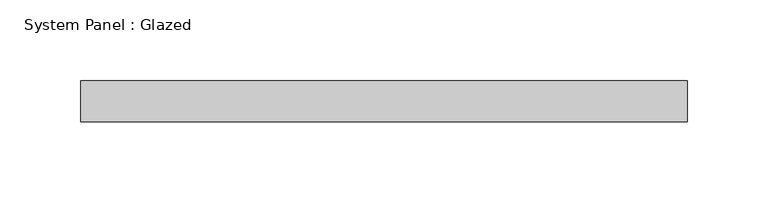
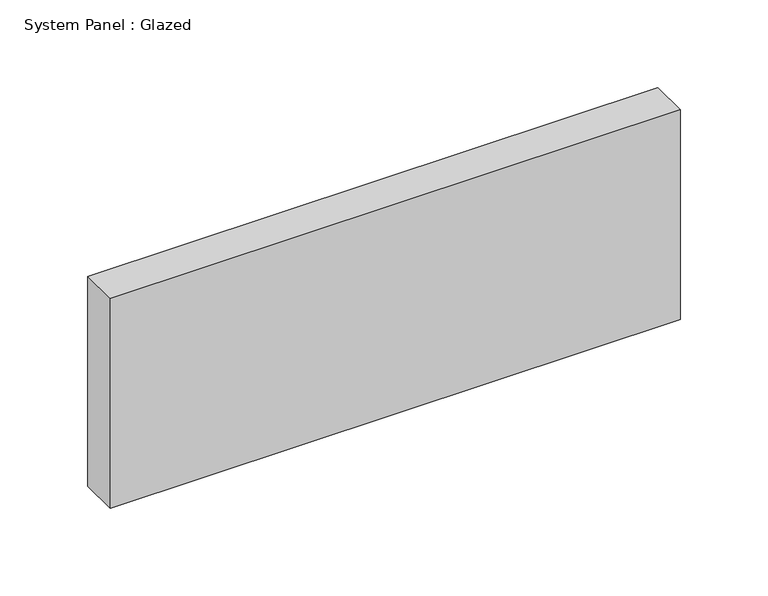
"""IFC4 building model written with IfcOpenShell, lengths in millimetres: plate geometry, System Panel : Glazed."""

from ifc_helpers import new_model, si_unit, origin, origin_with_axes, place, context, project, spatial, polyline, outline, extrude, source, transform, mapped, element, save


def system_panel_glazed_a64eeae2(model_context):
    return source(origin(), model_context, "Body", "SweptSolid", [
        extrude(outline(polyline([(187.5766464, 19.05), (-187.5766464, 19.05), (-187.5766464, 44.45), (187.5766464, 44.45), (187.5766464, 19.05)])), origin_with_axes(), (0.0, 0.0, 1.0), 146.05),
    ])


if __name__ == "__main__":
    model = new_model("IFC4")
    model_context = context("Model", 3, world=origin())
    ifc_project = project(units=[si_unit("LENGTHUNIT", "METRE", prefix="MILLI")], contexts=[model_context])
    site = spatial("IfcSite", under=ifc_project)
    building = spatial("IfcBuilding", under=site)
    placement = place(None, origin())
    system_panel_glazed_shape = system_panel_glazed_a64eeae2(model_context)
    element("IfcPlate", 1, ObjectType="System Panel : Glazed", at=placement, inside=building, context=model_context, shape_type="MappedRepresentation", body=[
        mapped(system_panel_glazed_shape, transform((0.0, 0.0, 0.0), x_axis=(1.0, 0.0, 0.0), y_axis=(0.0, 1.0, 0.0), z_axis=(0.0, 0.0, 1.0))),
    ])
    save(model, "model.ifc")

# Revit data of these elements
# Type "System Panel : Glazed"
#   Construction Type Id = "GSP4R"
#   Analytic Construction = "1/8 in Pilkington single glazing"
#   Visual Light Transmittance = 0.9
#   Solar Heat Gain Coefficient = 0.86
#   Heat Transfer Coefficient (U) = 1.18115 BTU/(h·ft²·°F)
#   Define Thermal Properties by = 1
# Element 1 (IfcPlate, "System Panel : Glazed")
#   Materials on its faces: "Glass"
# Materials
#   "Glass": class "Glass", colour RGB 0 128 192, transparency 0.75, Description = "Soda Lime Glass", Cost = 0
